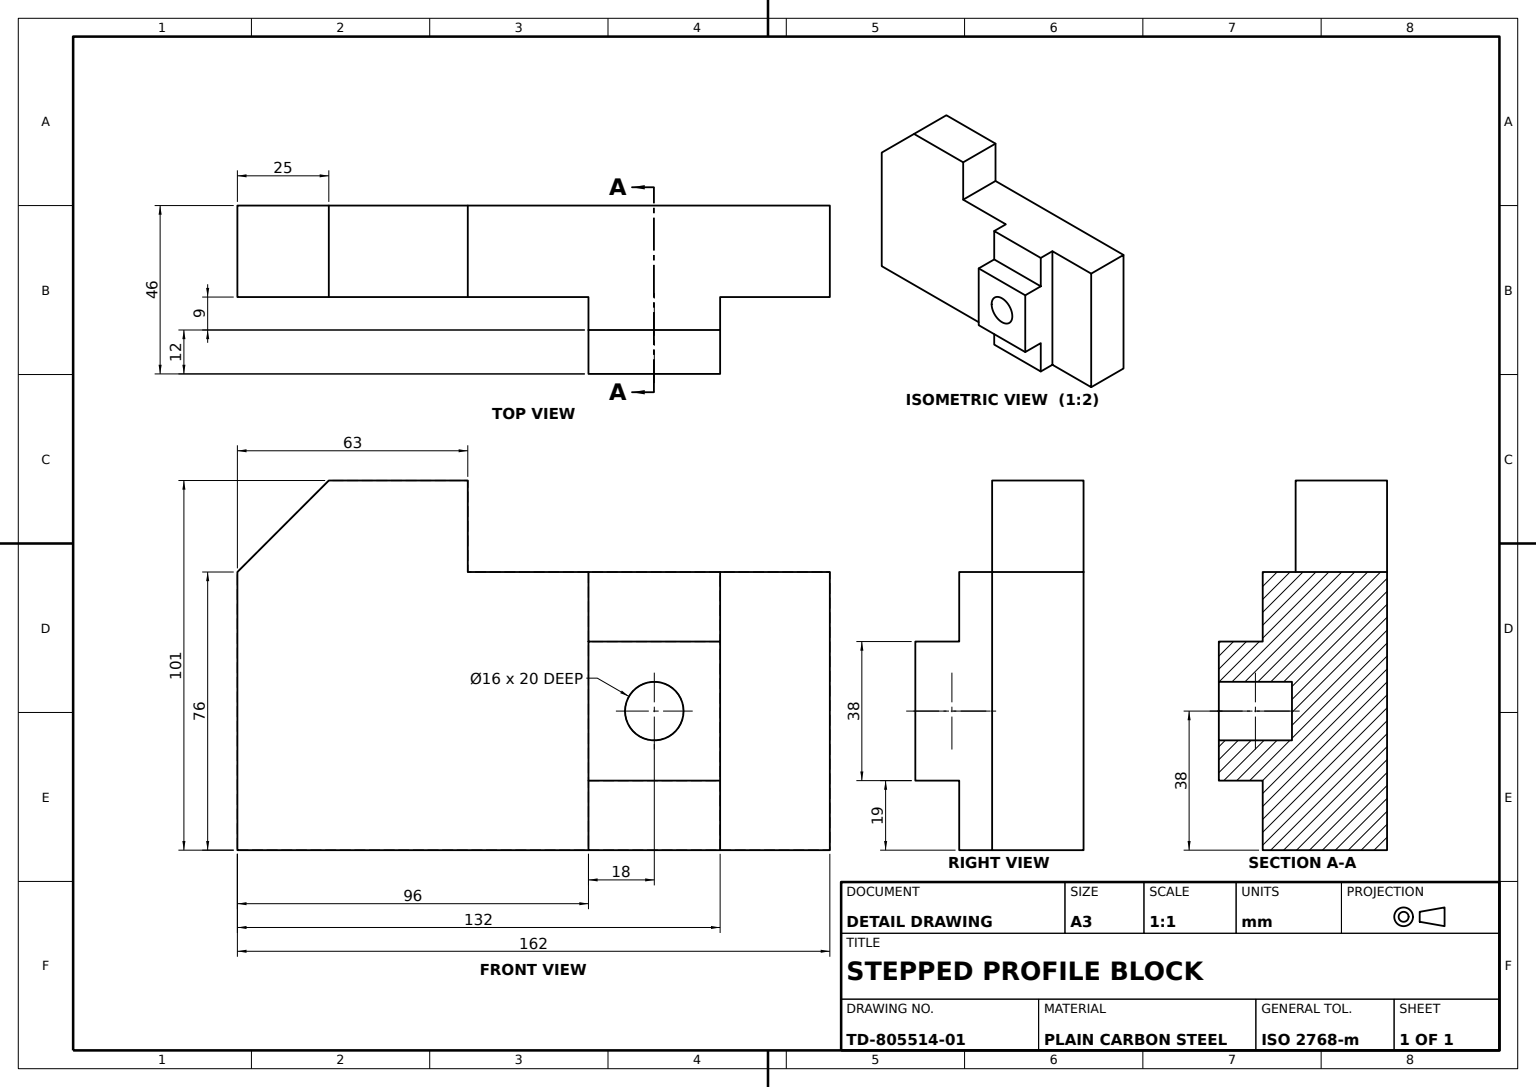
SolidWorks part; units mm, degrees
material "Plain Carbon Steel"
ref_plane "Front Plane" through (0, 0, 0) normal (0, 0, 1) x (1, 0, 0)
ref_plane "Top Plane" through (0, 0, 0) normal (0, 1, 0) x (1, 0, 0)
ref_plane "Right Plane" through (0, 0, 0) normal (1, 0, 0) x (0, 0, -1)
sketch "Base Profile Sketch" plane through (0, 0, 0) normal (0, 0, 1) x (1, 0, 0)
  line L0 (0, 0) -> (162, 0)
  line L1 (162, 0) -> (162, 76)
  line L2 (162, 76) -> (25, 76)
  line L3 (0, 0) -> (0, 51)
  line L4 (0, 51) -> (0, 76)
  line L5 (0, 76) -> (25, 76)
  dimension "D1" = 25
  dimension "D2" = 162
  dimension "D3" = 51
extrude "Base Block" add sketch "Base Profile Sketch" along normal blind 25
sketch "Side Block Sketch" plane through (0, 0, 25) normal (0, 0, 1) x (1, 0, 0)
  line L0 (0, 76) -> (0, 0) construction
  line L1 (162, 76) -> (0, 76) construction
  line L2 (63, 76) -> (63, 101)
  line L3 (63, 101) -> (25, 101)
  line L4 (25, 101) -> (0, 76)
  line L5 (0, 76) -> (25, 76)
  line L6 (25, 76) -> (63, 76)
  dimension "D1" = 25
  dimension "D2" = 63
extrude "Side Block" add sketch "Side Block Sketch" against normal blind 25
sketch "Pad Sketch" plane through (0, 0, 25) normal (0, 0, 1) x (1, 0, 0)
  line L0 (0, 76) -> (0, 0) construction
  line L1 (0, 0) -> (162, 0) construction
  line L2 (96, 0) -> (96, 76)
  line L3 (162, 76) -> (63, 76) construction
  line L4 (96, 76) -> (132, 76)
  line L5 (132, 76) -> (132, 0)
  line L6 (132, 0) -> (96, 0)
  dimension "D1" = 96
  dimension "D2" = 132
extrude "Mounting Pad" add sketch "Pad Sketch" along normal blind 9
sketch "Lug Boss Sketch" plane through (0, 0, 34) normal (0, 0, 1) x (1, 0, 0)
  line L0 (96, 0) -> (132, 0) construction
  line L1 (96, 76) -> (96, 0) construction
  line L2 (96, 57) -> (132, 57)
  line L3 (132, 0) -> (132, 76) construction
  line L4 (132, 57) -> (132, 19)
  line L5 (132, 19) -> (96, 19)
  line L6 (96, 76) -> (96, 0) construction
  line L7 (96, 19) -> (96, 57)
  dimension "D1" = 19
  dimension "D2" = 57
extrude "Lug Boss" add sketch "Lug Boss Sketch" along normal blind 12
sketch "Hole Sketch Ø16" plane through (0, 0, 46) normal (0, 0, 1) x (1, 0, 0)
  line L0 (96, 57) -> (96, 19) construction
  line L1 (96, 19) -> (132, 19) construction
  circle A0 centre (114, 38) radius 8
  dimension "D1" = 16
  dimension "D2" = 16
  dimension "D3" = 18
  dimension "D4" = 19
extrude "Hole Ø16" cut sketch "Hole Sketch Ø16" against normal blind 20
